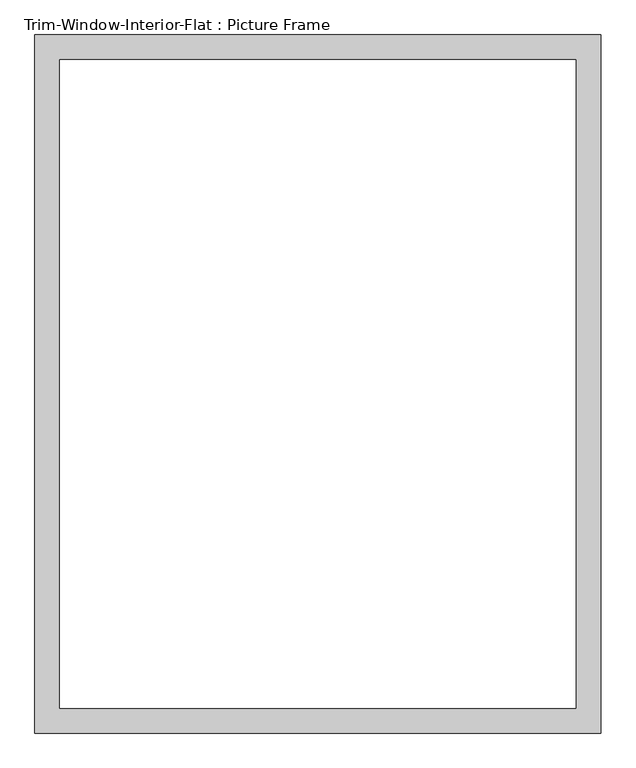
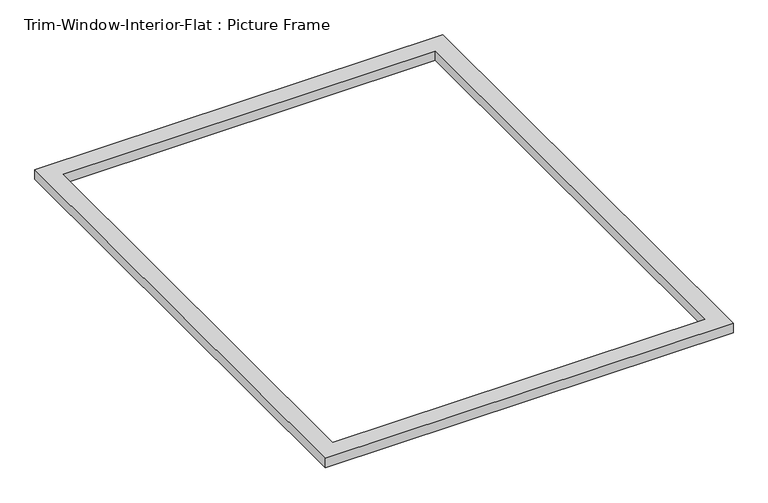
"""IFC4 building model written with IfcOpenShell, lengths in millimetres: proxy geometry, Trim-Window-Interior-Flat : Picture Frame."""

from ifc_helpers import new_model, si_unit, origin, origin_with_axes, place, context, project, spatial, polyline, outline, extrude, source, transform, mapped, element, save


def trim_window_interior_flat_picture_frame_1906adc9(model_context):
    return source(origin(), model_context, "Body", "SweptSolid", [
        extrude(outline(polyline([(654.05, -44.45), (-654.05, -44.45), (-654.05, 1568.45), (654.05, 1568.45), (654.05, -44.45)]), holes=[polyline([(596.9, 12.7), (596.9, 1511.3), (-596.9, 1511.3), (-596.9, 12.7), (596.9, 12.7)])]), origin_with_axes(), (0.0, 0.0, 1.0), 31.75),
    ])


if __name__ == "__main__":
    model = new_model("IFC4")
    model_context = context("Model", 3, world=origin())
    ifc_project = project(units=[si_unit("LENGTHUNIT", "METRE", prefix="MILLI")], contexts=[model_context])
    site = spatial("IfcSite", under=ifc_project)
    building = spatial("IfcBuilding", under=site)
    placement = place(None, origin())
    trim_window_interior_flat_picture_frame_shape = trim_window_interior_flat_picture_frame_1906adc9(model_context)
    element("IfcBuildingElementProxy", 1, Name="Trim-Window-Interior-Flat : Picture Frame", ObjectType="Trim-Window-Interior-Flat : Picture Frame", at=placement, inside=building, context=model_context, shape_type="MappedRepresentation", body=[
        mapped(trim_window_interior_flat_picture_frame_shape, transform((0.0, 0.0, 0.0), x_axis=(1.0, 0.0, 0.0), y_axis=(0.0, 1.0, 0.0), z_axis=(0.0, 0.0, 1.0))),
    ])
    save(model, "model.ifc")

# Revit data of these elements
# Type "Trim-Window-Interior-Flat : Picture Frame"
#   Trim Thickness_Picture Frame = 0' - 1 1/4"
#   Trim Width = 0' - 2 1/4"
#   Trim Thickness_with Sill = 0' - 0 3/4"
#   Sill Thickness = 0' - 1 1/4"
#   Opening Width [instance default] = 2' - 0"
#   Opening Height [instance default] = 3' - 0"
#   Default Elevation = 4' - 0"
#   Sill = no
#   Picture Frame = yes
#   Trim Material [instance default] = none
# Element 1 (IfcBuildingElementProxy, "Trim-Window-Interior-Flat : Picture Frame")
#   Opening Width = 4' - 0"
#   Opening Height = 5' - 0"
#   Trim Material = Wood - Stained
#   Materials on its faces: "Wood - Stained"
# Materials
#   "Wood - Stained": class "Wood", colour RGB 224 178 126, transparency 0, Cost = 0
